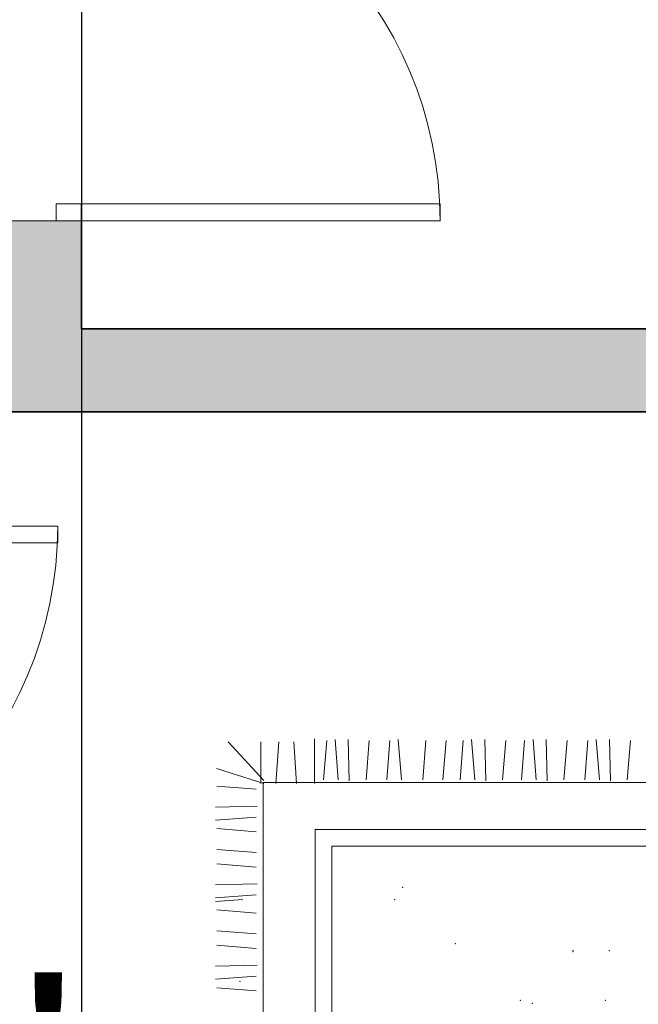
# Model space of a CAD drawing. Units: inches. Extents: x 1763 to 2368, y 1500 to 2097.
# Tile 15 of 24: x 2079 to 2117, y 1797 to 1856. Entities that reach past the tile are written whole.
import ezdxf

# ---------------------------------------------------------------- set-up
doc = ezdxf.new("R2010")
doc.units = ezdxf.units.IN
for name, color, linetype, lineweight in [('A-ANNO-DIMS', 2, 'Continuous', 18), ('A-DOOR', 4, 'Continuous', 18), ('A-FURN', 8, 'Continuous', 18), ('A-WALL', 7, 'Continuous', 35), ('A-WALL-PATT', 7, 'Continuous', 13)]:
    doc.layers.add(name, color=color, linetype=linetype, lineweight=lineweight)
doc.styles.get("Standard").update_dxf_attribs({"font": 'arial.ttf'})
doc.dimstyles.new('ISO-25', dxfattribs={"dimtxt": 12.5, "dimasz": 2.5, "dimexe": 1.25, "dimexo": 0.625, "dimtad": 1, "dimdec": 0, "dimlunit": 4, "dimtxsty": 'Standard', "dimblk": 'ARCHTICK', "dimcen": 2.5, "dimclrd": 3, "dimclrt": 4, "dimadec": 0, "dimazin": 0, "dimtfac": 1, "dimtdec": 0, "dimtmove": 0, "dimatfit": 3, "dimfxl": 1, "dimarcsym": 0})

# ---------------------------------------------------------------- blocks, each defined once
blk = doc.blocks.new('A$C77DF40FE')
for p, q in [((0.1002397472184384, 1.888474420258717), (0.1002397472184384, 0.0935002162950696)), ((0.1852251112431986, 1.811603981208463), (0.1852251112431986, 0.1869505834038136)), ((0.2152251112420345, 1.781603981209627), (0.2152251112420345, 0.2169505834026495)), ((0.0247191405724152, 0.7548065529699671), (0.0955424953790498, 0.7491367263210122)), ((0.0226663125285995, 0.7171728351022466), (0.097390093105787, 0.7188162710299367)), ((0.0226663125285995, 0.6933436513354537), (0.0957477256961283, 0.6990955860601389)), ((0.0247191405724152, 0.6782658048541635), (0.0955424953790498, 0.6725959782124847)), ((0.0247191405724152, 0.6408332608843921), (0.0955424953790498, 0.6351634342354373)), ((0.0226663125285995, 0.6031995430166717), (0.097390093105787, 0.6048429789443617)), ((0.0226663125285995, 0.5793703592498787), (0.0957477256961283, 0.585122293974564)), ((0.0247191405724152, 0.5642925127685885), (0.0955424953790498, 0.5586226861269097)), ((0.0247191405724152, 0.530116254944005), (0.0955424953790498, 0.5244464282950503)), ((0.0226663125285995, 0.4924825370762847), (0.097390093105787, 0.4941259730039747)), ((0.0226663125285995, 0.4686533533094917), (0.0957477256961283, 0.474405288034177)), ((0.0247191405724152, 0.4535755068282015), (0.0955424953790498, 0.4479056801865227)), ((0.0247191405724152, 0.4226553530897946), (0.0955424953790498, 0.4169855264408398)), ((0.0247191405724152, 0.3863853563088924), (0.0955424953790498, 0.3807155296672135)), ((0.0226663125285995, 0.336688923627662), (0.0957477256961283, 0.3424408583450713)), ((0.0247191405724152, 0.3216110771463718), (0.0955424953790498, 0.3159412504974171)), ((0.0247191405724152, 0.2841785331693245), (0.0955424953790498, 0.2785087065203697)), ((0.0226663125285995, 0.2465448153016041), (0.097390093105787, 0.2481882512365701)), ((0.0226663125285995, 0.2227156315420871), (0.0957477256961283, 0.2284675662594964)), ((0.2152251112420345, 0.2169505834026495), (0.3112043679720955, 0.2169505834026495)), ((0.3112043679720955, 0.2169505834026495), (1.613872679183259, 0.2169505834026495)), ((0.0247191405724152, 0.2076377850607969), (0.0955424953790498, 0.2019679584118421)), ((0.1018629931495525, 0.1856925320898881), (0.0215859625604935, 0.1856925320898881)), ((0.1852251112431986, 0.1869505834038136), (0.3112043679720955, 0.1869505834038136)), ((0.3112043679720955, 0.1869505834038136), (1.643872679182095, 0.1869505834038136)), ((0.1018629931495525, 0.153544231550768), (0.0269378679586225, 0.1481852358119795)), ((0.1018629931495525, 0.1160369352728594), (0.0269378679586225, 0.1213930940648424)), ((0.0965110877514235, 0.0946037892645109), (0.0269378679586225, 0.0303071881862707)), ((0.1018629931495525, 0.0892447935257224), (0.0269378679586225, 0.0892447935257224)), ((0.1018629931495525, 0.0946037892645109), (0.0751034661589074, 0.0088740421779221)), ((0.1002397472184384, 0.0935002162950696), (0.3112043679720955, 0.0935002162950696)), ((0.3112043679720955, 0.0935002162950696), (1.015486722324567, 0.0935002162950696)), ((0.1069568759485264, 0.0096009220796986), (0.1126267025974812, 0.0804242768863333)), ((0.1445905938162468, 0.007548094035883), (0.1429471578885568, 0.0822718746130704)), ((0.1684197775830398, 0.007548094035883), (0.1626678428583546, 0.0806295072034118)), ((0.18349762406433, 0.0096009220796986), (0.1891674507060088, 0.0804242768863333)), ((0.2209301680341014, 0.0096009220796986), (0.2265999946830561, 0.0804242768863333)), ((0.2469813674761099, 0.0096009220796986), (0.2526511941250646, 0.0804242768863333)), ((0.2846150853438303, 0.007548094035883), (0.2829716494161403, 0.0822718746130704)), ((0.3084442691106233, 0.007548094035883), (0.302692334385938, 0.0806295072034118)), ((0.3301377238531131, 0.0096009220796986), (0.3358075505020679, 0.0804242768863333)), ((0.3675702678301604, 0.0096009220796986), (0.3732400944791152, 0.0804242768863333)), ((0.3936214672721689, 0.0096009220796986), (0.3992912939211237, 0.0804242768863333)), ((0.4312551851398894, 0.007548094035883), (0.4296117492049234, 0.0822718746130704)), ((0.4550843688994064, 0.007548094035883), (0.4493324341819971, 0.0806295072034118)), ((0.4701622153806966, 0.0096009220796986), (0.4758320420296514, 0.0804242768863333)), ((0.3150598773718229, 0.007548094035883), (0.3112043679720955, 0.0565344072383596))]:
    blk.add_line(p, q)
for p in [(0.4034435357025359, 0.7168515314842808), (0.4931307316510356, 0.7095942980013206), (0.4034435357025359, 0.6511853100746521), (0.4055166808320792, 0.6512242505123141), (0.4983588332761429, 0.5782229147444014), (0.4931307316510356, 0.5563730709764059), (0.3909143693745136, 0.439633238442184), (0.2894910708273528, 0.3447820589062758), (0.3113944469878334, 0.3301895798358601), (0.4588475937125623, 0.0512694676363026)]:
    blk.add_point(p)
blk = doc.blocks.new('*U3')
for p, q in [((0, 0), (-1e-16, -5.999999999999999)), ((40, -6e-16), (40, -6))]:
    blk.add_line(p, q)
blk.add_lwpolyline([(0, 0), (5.6e-15, 40), (1.750000000000007, 40), (1.749999999999998, -7e-16)], close=True)
blk.add_arc((0, 0), 40, 0, 90)
blk = doc.blocks.new('_ArchTick')
at = {"color": 0, "linetype": 'ByBlock', "const_width": 0.15}
blk.add_lwpolyline([(-0.5, -0.5), (0.5, 0.5)], dxfattribs=at)
blk = doc.blocks.new('*D27')
at = {"layer": 'A-ANNO-DIMS', "color": 0, "lineweight": -2, "transparency": 16777216}
for p, q in [((1853.713196592648, 1795.957703707508), (1853.713196592648, 1781.682703707508)), ((1944.713196592648, 1795.957703707508), (1944.713196592648, 1781.682703707508))]:
    blk.add_line(p, q, dxfattribs=at)
at = {"layer": 'A-ANNO-DIMS', "color": 3, "lineweight": -2, "transparency": 16777216}
for p, q in [((1853.713196592648, 1782.932703707508), (1944.713196592648, 1782.932703707508)), ((1944.713196592648, 1782.932703707508), (2085.85235075363, 1782.932703707508))]:
    blk.add_line(p, q, dxfattribs=at)
at = {"layer": 'Defpoints', "color": 0, "transparency": 16777216}
for p in [(1853.713196592648, 1796.582703707508), (1944.713196592648, 1796.582703707508), (1944.713196592648, 1782.932703707508)]:
    blk.add_point(p, dxfattribs=at)
at = {"layer": 'A-ANNO-DIMS', "color": 3, "lineweight": -2, "transparency": 16777216, "xscale": 2.5, "yscale": 2.5, "zscale": 2.5, "rotation": 180}
blk.add_blockref('_ArchTick', (1853.713196592648, 1782.932703707508), dxfattribs=at)
at = {"layer": 'A-ANNO-DIMS', "color": 3, "lineweight": -2, "transparency": 16777216, "xscale": 2.5, "yscale": 2.5, "zscale": 2.5}
blk.add_blockref('_ArchTick', (1944.713196592648, 1782.932703707508), dxfattribs=at)
at = {"layer": 'A-ANNO-DIMS', "color": 4, "transparency": 16777216, "insert": (2016.532773673139, 1790.020868782542), "char_height": 12.5, "attachment_point": 5}
blk.add_mtext('DINING SET 7\'-7"', dxfattribs=at)
blk = doc.blocks.new('*D62')
at = {"layer": 'A-ANNO-DIMS', "color": 0, "lineweight": -2, "transparency": 16777216}
for p, q in [((2083.09181, 1980.647691), (2083.09181, 1509.906119)), ((2120.612101, 1980.647691), (2120.612101, 1509.906119))]:
    blk.add_line(p, q, dxfattribs=at)
at = {"layer": 'A-ANNO-DIMS', "color": 3, "lineweight": -2, "transparency": 16777216}
for p, q in [((2083.09181, 1511.156119), (2120.612101, 1511.156119)), ((2120.612101, 1511.156119), (2186.708622145976, 1511.156119))]:
    blk.add_line(p, q, dxfattribs=at)
at = {"layer": 'Defpoints', "color": 0, "transparency": 16777216}
for p in [(2083.09181, 1981.272691), (2120.612101, 1981.272691), (2120.612101, 1511.156119)]:
    blk.add_point(p, dxfattribs=at)
at = {"layer": 'A-ANNO-DIMS', "color": 3, "lineweight": -2, "transparency": 16777216, "xscale": 2.5, "yscale": 2.5, "zscale": 2.5, "rotation": 180}
blk.add_blockref('_ArchTick', (2083.09181, 1511.156119), dxfattribs=at)
at = {"layer": 'A-ANNO-DIMS', "color": 3, "lineweight": -2, "transparency": 16777216, "xscale": 2.5, "yscale": 2.5, "zscale": 2.5}
blk.add_blockref('_ArchTick', (2120.612101, 1511.156119), dxfattribs=at)
at = {"layer": 'A-ANNO-DIMS', "color": 4, "transparency": 16777216, "insert": (2154.910361572988, 1518.248547376535), "char_height": 12.5, "attachment_point": 5}
blk.add_mtext('3\'-1 1/2"', dxfattribs=at)
blk = doc.blocks.new('*D71')
at = {"layer": 'A-ANNO-DIMS', "color": 0, "lineweight": -2, "transparency": 16777216}
for p, q in [((2049.685769, 1879.647691), (2049.685769, 1509.906119)), ((2072.784807, 1879.647691), (2072.784807, 1509.906119))]:
    blk.add_line(p, q, dxfattribs=at)
at = {"layer": 'A-ANNO-DIMS', "color": 3, "lineweight": -2, "transparency": 16777216}
for p, q in [((2049.685769, 1511.156119), (2072.784807, 1511.156119)), ((2072.784807, 1511.156119), (2118.298108500682, 1511.156119))]:
    blk.add_line(p, q, dxfattribs=at)
at = {"layer": 'Defpoints', "color": 0, "transparency": 16777216}
for p in [(2049.685769, 1880.272691), (2072.784807, 1880.272691), (2072.784807, 1511.156119)]:
    blk.add_point(p, dxfattribs=at)
at = {"layer": 'A-ANNO-DIMS', "color": 3, "lineweight": -2, "transparency": 16777216, "xscale": 2.5, "yscale": 2.5, "zscale": 2.5, "rotation": 180}
blk.add_blockref('_ArchTick', (2049.685769, 1511.156119), dxfattribs=at)
at = {"layer": 'A-ANNO-DIMS', "color": 3, "lineweight": -2, "transparency": 16777216, "xscale": 2.5, "yscale": 2.5, "zscale": 2.5}
blk.add_blockref('_ArchTick', (2072.784807, 1511.156119), dxfattribs=at)
at = {"layer": 'A-ANNO-DIMS', "color": 4, "transparency": 16777216, "insert": (2096.791457750341, 1518.056698809004), "char_height": 12.5, "attachment_point": 5}
blk.add_mtext('1\'-11"', dxfattribs=at)

msp = doc.modelspace()

# ---------------------------------------------------------------- hatches: boundary and pattern name
at = {"layer": 'A-WALL-PATT'}
h = msp.add_hatch(color=256, dxfattribs=at)
h.dxf.hatch_style = 1
h.paths.add_polyline_path([(1838.091809557101, 2034.272690883634), (1838.091809557101, 2043.272690883634), (1829.091809557101, 2043.272690883634), (1829.091809557101, 1953.387436665241), (1838.091809557101, 1953.387436665241)])
h.paths.add_polyline_path([(1838.091809557101, 1913.100906919557), (1829.091809557101, 1913.100906919557), (1829.091809557101, 1862.201751012257), (1838.091809557101, 1862.201751012257)])
h.paths.add_polyline_path([(1838.091809557101, 1825.58961200371), (1829.091809557101, 1825.58961200371), (1829.091809557101, 1738.643388462881), (1838.091809557101, 1738.643388462881)])
h.paths.add_polyline_path([(1895.591809557102, 1885.272690883634), (1838.091809557101, 1885.272690883634), (1838.091809557101, 1880.272690883634), (1895.591809557102, 1880.272690883634)])
h.paths.add_polyline_path([(1857.388795027446, 1784.272690883634), (1838.091809557101, 1784.272690883634), (1838.091809557101, 1779.272690883634), (1857.388795027446, 1779.272690883634)])
h.paths.add_polyline_path([(1958.091809557101, 1981.272690883634), (1971.455231199137, 1981.272690883634), (1971.455231199137, 1986.272690883634), (1968.567697615106, 1986.272690883634), (1958.091809557101, 1986.272690883634), (1953.091809557101, 1986.272690883634), (1927.390355781482, 1986.272690883634), (1927.390355781482, 1981.272690883634), (1953.091809557102, 1981.272690883634), (1953.091809557102, 1885.272690883634), (1932.013525308711, 1885.272690883634), (1932.013525308711, 1880.272690883634), (1959.134211901633, 1880.272690883634), (1959.134211901633, 1883.737546537067), (1959.134211901633, 1885.272690883634), (1958.091809557101, 1885.272690883634)])
h.paths.add_polyline_path([(2018.091809557102, 1981.272690883634), (2031.018823922628, 1981.272690883634), (2031.018823922628, 1986.272690883634), (2018.091809557102, 1986.272690883634), (2013.091809557101, 1986.272690883634), (2001.2328901763, 1986.272690883634), (2001.2328901763, 1981.272690883634), (2013.091809557101, 1981.272690883634), (2013.091809557101, 1885.272690883634), (1982.182180879804, 1885.272690883634, -0.0166285960272348), (1982.233249591189, 1883.737546537067), (1982.233249591189, 1880.272690883634), (2049.685769014253, 1880.272690883634), (2049.685769014253, 1883.737546537067, -0.0166285960272329), (2049.736837725638, 1885.272690883634), (2018.091809557102, 1885.272690883634)])
h.paths.add_polyline_path([(2083.091809557101, 1981.272690883633), (2120.612101449853, 1981.272690883633), (2120.612101449853, 1986.272690883634), (2083.091809557101, 1986.272690883634), (2078.091809557101, 1986.272690883634), (2063.142597715185, 1986.272690883634), (2063.142597715185, 1981.272690883634), (2078.091809557101, 1981.272690883634), (2078.091809557101, 1885.272690883634), (2072.784806703809, 1885.272690883634), (2072.784806703809, 1883.737546537067), (2072.784806703809, 1880.272690883634), (2078.091809557101, 1880.272690883634), (2078.091809557101, 1866.867159403521), (2081.556665210535, 1866.867159403521, -0.0166285960272329), (2083.091809557101, 1866.816090692136)])
h.paths.add_polyline_path([(1871.675401748104, 1635.272690883634), (1838.091809557101, 1635.272690883634), (1838.091809557101, 1626.272690883634), (1871.675401748104, 1626.272690883634)], flags=17)
h.paths.add_polyline_path([(2100.577130801176, 1688.272690883634), (2060.091809557102, 1688.272690883634), (2060.091809557102, 1679.272690883634), (2100.577130801176, 1679.272690883634)], flags=17)
h.paths.add_polyline_path([(2180.091809557101, 1688.272690883634), (2148.743529320587, 1688.272690883634), (2148.743529320587, 1679.272690883634), (2180.091809557101, 1679.272690883634)], flags=17)
h.paths.add_polyline_path([(2189.091809557101, 1746.219079973147), (2180.091809557101, 1746.219079973147), (2180.091809557101, 1743.41673524497), (2180.123283967846, 1743.41673524497), (2180.123283967846, 1726.723261858881), (2180.091809557101, 1572.272690883634), (2034.906803433656, 1572.272690883634), (2034.906803433656, 1565.600894774026), (2034.906803433656, 1563.272690883634), (2189.091809557101, 1563.272690883634)])
h.paths.add_polyline_path([(2060.091809557102, 1802.347155552507, -0.0166285960272347), (2058.556665210535, 1802.296086841122), (2055.091809557101, 1802.296086841122), (2055.091809557101, 1635.272690883634), (2042.484481853934, 1635.272690883634), (2042.484481853934, 1629.737546537067), (2042.484481853934, 1626.272690883634), (2055.091809557101, 1626.272690883634), (2055.091809557101, 1599.272690883634), (2040.268709306729, 1599.272690883634), (2040.268709306729, 1590.272690883634), (2060.091809557102, 1590.272690883634)])
h.paths.add_polyline_path([(2019.385444164378, 1629.737546537071, -0.0605692182813801), (2020.058431839583, 1635.272690883634), (1995.091809557101, 1635.272690883634), (1990.091809557101, 1635.272690883634), (1927.074869319207, 1635.272690883634), (1927.074869319207, 1626.272690883634), (1990.091809557101, 1626.272690883634), (1990.091809557102, 1590.272690883634), (1995.091809557101, 1590.272690883634), (2005.195459372391, 1590.272690883634), (2005.195459372391, 1599.272690883634), (1995.091809557101, 1599.272690883634), (1995.091809557101, 1626.272690883634), (2019.385444164378, 1626.272690883634)])
edge = h.paths.add_edge_path()
edge.add_line((2180.091809557101, 1837.272690883634), (2167.198417694339, 1837.272690883634))
edge.add_spline(control_points=[(2167.198417694823, 1837.272690883674), (2167.1907827488, 1837.271431447654), (2167.183204353112, 1837.271421440364), (2167.175683403496, 1837.272690883654)], knot_values=[168.9554928085609, 168.9554928085609, 168.9554928085609, 168.9554928085609, 169.0658706879006, 169.0658706887506, 169.0658706887506, 169.0658706887506], degree=3, periodic=0)
edge.add_spline(control_points=[(2167.175683403438, 1837.272690883663), (2166.556253545484, 1837.377242984508), (2166.326495733136, 1846.160649987724), (2165.707502931977, 1846.244137993658)], knot_values=[159.864705322856, 159.8647053237059, 159.8647053237059, 159.8647053237059, 168.9554928094108, 168.9554928094108, 168.9554928094108, 168.9554928094108], degree=3, periodic=0)
edge.add_line((2167.122451608289, 1837.272690883634), (2163.159522476786, 1837.272690883634))
edge.add_spline(control_points=[(2163.159522482475, 1837.272690883686), (2163.15796606182, 1837.2726620788), (2163.156410184994, 1837.272662044343), (2163.15485485529, 1837.272690883634)], knot_values=[150.5371721295467, 150.5371721295467, 150.5371721295467, 150.5371721295467, 150.5537966479016, 150.5537966479139, 150.5537966479139, 150.5537966479139], degree=3, periodic=0)
edge.add_spline(control_points=[(2163.154854855289, 1837.272690883634), (2162.290043487653, 1837.288726420245), (2161.594386529693, 1846.231668717186), (2160.877825059406, 1846.244137993679)], knot_values=[141.2934262950179, 141.2934262950303, 141.2934262950303, 141.2934262950303, 150.5371721295591, 150.5371721295591, 150.5371721295591, 150.5371721295591], degree=3, periodic=0)
edge.add_line((2163.075401221166, 1837.272690883634), (2158.699619590683, 1837.272690883634))
edge.add_spline(control_points=[(2158.6996195907, 1837.272690883634), (2158.698397652875, 1837.272665391618), (2158.697175755076, 1837.272665420255), (2158.695953896478, 1837.272690883674)], knot_values=[132.0335441852708, 132.0335441852708, 132.0335441852708, 132.0335441852771, 132.0491510388534, 132.0491510388534, 132.0491510388534, 132.0491510388534], degree=3, periodic=0)
edge.add_spline(control_points=[(2158.695953896478, 1837.272690883674), (2157.971966468073, 1837.287778714179), (2157.261742058153, 1846.232799164874), (2156.393385429706, 1846.244137993689)], knot_values=[122.7860209386129, 122.7860209386129, 122.7860209386129, 122.7860209386129, 132.0335441852594, 132.0335441852594, 132.0335441852594, 132.0335441852708], degree=3, periodic=0)
edge.add_line((2158.629450057908, 1837.272690883634), (2153.839354197273, 1837.272690883634))
edge.add_spline(control_points=[(2153.839354197267, 1837.272690883633), (2153.831393241206, 1837.271421595935), (2153.823483829624, 1837.271411470755), (2153.815626850732, 1837.272690883634)], knot_values=[113.4515845582001, 113.4515845582001, 113.4515845582001, 113.4515845582001, 113.5621029574639, 113.5621029574639, 113.5621029574639, 113.5621029574668], degree=3, periodic=0)
edge.add_spline(control_points=[(2153.815626850732, 1837.272690883634), (2153.16997926524, 1837.3778266931), (2152.878395890465, 1846.19087494863), (2152.403814355283, 1846.244137993689)], knot_values=[0, 0, 0, 0, 9.081854313454823, 9.081854313454823, 9.081854313454823, 9.081854313454823], degree=3, periodic=0)
edge.add_line((2153.760174359353, 1837.272690883634), (2150.390681228399, 1837.272690883634))
edge.add_spline(control_points=[(2150.390681228397, 1837.272690883634), (2150.380731407352, 1837.271531119858), (2150.370755552885, 1837.271539860845), (2150.360754310833, 1837.272690883655)], knot_values=[95.0693824194044, 95.0693824194044, 95.0693824194044, 95.06938241940794, 95.17519011295934, 95.17519011295934, 95.17519011295934, 95.17519011295934], degree=3, periodic=0)
edge.add_spline(control_points=[(2150.360754310833, 1837.272690883655), (2149.486911233016, 1837.373259724043), (2148.41925626668, 1846.194145922126), (2147.588575190972, 1846.244137993689)], knot_values=[85.8245986104526, 85.8245986104526, 85.8245986104526, 85.8245986104526, 95.06938241940442, 95.06938241940442, 95.06938241940442, 95.06938241940442], degree=3, periodic=0)
edge.add_line((2150.286144937881, 1837.272690883634), (2145.429521599744, 1837.272690883634))
edge.add_spline(control_points=[(2145.429521599744, 1837.272690883634), (2145.426173195383, 1837.272505952667), (2145.422821785984, 1837.272506511139), (2145.419467387339, 1837.272690883634)], knot_values=[76.50555885182466, 76.50555885182466, 76.50555885182466, 76.50555885182986, 76.54781121413636, 76.54781121413636, 76.54781121413636, 76.54781121413636], degree=3, periodic=0)
edge.add_spline(control_points=[(2145.419467387339, 1837.272690883634), (2144.683834601378, 1837.313124495274), (2143.804436376202, 1846.193948544996), (2142.947843667561, 1846.244137993688)], knot_values=[67.23944999382844, 67.23944999382844, 67.23944999382844, 67.23944999382844, 76.50555885179328, 76.50555885179328, 76.50555885179328, 76.50555885182465], degree=3, periodic=0)
edge.add_line((2145.353375417295, 1837.272690883634), (2134.569944747806, 1837.272690883634))
edge.add_spline(control_points=[(2134.56994474779, 1837.272690883634), (2134.566672918288, 1837.272498574207), (2134.563405957571, 1837.27249916596), (2134.560143779651, 1837.272690883636)], knot_values=[39.00146280124788, 39.00146280124788, 39.00146280124788, 39.00146280126319, 39.04510672327663, 39.04510672327663, 39.04510672327663, 39.04510672327663], degree=3, periodic=0)
edge.add_spline(control_points=[(2134.560143779651, 1837.272690883636), (2133.872211796742, 1837.313120536706), (2133.396974976361, 1845.853088067863), (2132.328029807564, 1846.244137993689)], knot_values=[29.79778030706209, 29.79778030706209, 29.79778030706209, 29.79778030706209, 39.00146280124655, 39.00146280124788, 39.00146280124788, 39.00146280124788], degree=3, periodic=0)
edge.add_line((2134.498286803723, 1837.272690883634), (2128.075271300648, 1837.272690883634))
edge.add_spline(control_points=[(2128.075271300648, 1837.272690883634), (2128.026285766884, 1837.259723584904), (2127.978195692325, 1837.26004073722), (2127.930927784897, 1837.272690883634)], knot_values=[19.48206652474599, 19.48206652474599, 19.48206652474599, 19.48206652474654, 19.86939583794397, 19.86939583794397, 19.86939583794397, 19.86939583794397], degree=3, periodic=0)
edge.add_spline(control_points=[(2125.013283184744, 1846.244137993688), (2126.164818330763, 1844.662568162717), (2126.821349600389, 1837.569643451595), (2127.930927784897, 1837.272690883634)], knot_values=[10.38980542113492, 10.3898054211352, 10.3898054211352, 10.3898054211352, 19.48206652474599, 19.48206652474599, 19.48206652474599, 19.48206652474599], degree=3, periodic=0)
edge.add_line((2127.930927784898, 1837.272690883634), (2083.091809557101, 1837.272690883634))
edge.add_line((2083.091809557101, 1837.272690883634), (2083.091809557101, 1843.768121713965))
edge.add_line((2083.091809557101, 1843.768121713965), (2081.556665210535, 1843.768121713965))
edge.add_line((2081.556665210535, 1843.768121713965), (2078.091809557101, 1843.768121713965))
edge.add_line((2078.091809557101, 1843.768121713965), (2078.091809557101, 1837.272690883634))
edge.add_line((2078.091809557101, 1837.272690883634), (2055.091809557101, 1837.272690883634))
edge.add_line((2055.091809557101, 1837.272690883634), (2055.091809557101, 1825.395124530677))
edge.add_line((2055.091809557101, 1825.395124530677), (2058.556665210535, 1825.395124530677))
edge.add_line((2058.556665210535, 1825.395124530677), (2060.091809557102, 1825.395124530677))
edge.add_line((2060.091809557102, 1825.395124530677), (2060.091809557102, 1832.272690883634))
edge.add_line((2060.091809557102, 1832.272690883634), (2122.436734598602, 1832.272690883634))
edge.add_spline(control_points=[(2122.436734598601, 1832.272690883634), (2122.727456143255, 1832.584305259818), (2123.008062474702, 1832.616792422395), (2123.275021713284, 1832.272690883634)], knot_values=[5.972032537224317, 5.972032537224317, 5.972032537224317, 5.972032537224317, 8.057258009602386, 8.057258009602837, 8.057258009602837, 8.057258009602837], degree=3, periodic=0)
edge.add_line((2123.275021713284, 1832.272690883634), (2137.951393308032, 1832.272690883634))
edge.add_spline(control_points=[(2137.951393307966, 1832.272690883629), (2137.961042543445, 1832.274026104781), (2137.970676309981, 1832.27403826157), (2137.980294423909, 1832.272690883634)], knot_values=[53.92686179676418, 53.92686179676418, 53.92686179676418, 53.92686179676418, 54.03007548000314, 54.03007548000314, 54.03007548000314, 54.03007548000601], degree=3, periodic=0)
edge.add_spline(control_points=[(2139.715582741171, 1825.016325920323), (2139.281482802356, 1825.062086475526), (2138.671282749905, 1832.175892027703), (2137.98029442391, 1832.272690883634)], knot_values=[54.03007548000314, 54.03007548000314, 54.03007548000314, 54.03007548000314, 61.44519353062353, 61.44519353062641, 61.44519353062641, 61.44519353062641], degree=3, periodic=0)
edge.add_line((2138.045183132032, 1832.272690883634), (2140.961787078569, 1832.272690883634))
edge.add_spline(control_points=[(2140.96178707854, 1832.272690883628), (2140.970606368947, 1832.274440590632), (2140.979501539198, 1832.27442261757), (2140.988470957723, 1832.272690883634)], knot_values=[68.85418231261454, 68.85418231261454, 68.85418231261454, 68.85418231280003, 68.97123731673409, 68.97123731673409, 68.97123731673409, 68.97123731673409], degree=3, periodic=0)
edge.add_spline(control_points=[(2143.18986511145, 1825.016325920314), (2142.436495288906, 1825.065396856983), (2141.561146249046, 1832.16212393513), (2140.988470957723, 1832.272690883634)], knot_values=[68.9712373167341, 68.97123731708082, 68.97123731708082, 68.97123731708082, 76.44491114487315, 76.44491114487315, 76.44491114487315, 76.44491114487315], degree=3, periodic=0)
edge.add_line((2141.040932085754, 1832.272690883634), (2145.429521599744, 1832.272690883634))
edge.add_spline(control_points=[(2145.429521599742, 1832.272690883634), (2145.43886220747, 1832.273579662711), (2145.448227241903, 1832.27357314134), (2145.457616067813, 1832.272690883634)], knot_values=[84.03904662338796, 84.03904662338796, 84.03904662338796, 84.03904662338971, 84.12404068496751, 84.12404068496751, 84.12404068496751, 84.12404068496751], degree=3, periodic=0)
edge.add_spline(control_points=[(2148.107765738118, 1825.016325920317), (2147.340420200817, 1825.019697773855), (2146.30265295, 1832.193283691691), (2145.457616067813, 1832.272690883634)], knot_values=[84.12404068496751, 84.12404068496751, 84.12404068496751, 84.12404068496751, 91.77389142141917, 91.77389142141917, 91.77389142141917, 91.77389142141917], degree=3, periodic=0)
edge.add_line((2145.537886823607, 1832.272690883634), (2150.392945902062, 1832.272690883634))
edge.add_spline(control_points=[(2150.392945902064, 1832.272690883634), (2150.41883348599, 1832.27702102203), (2150.445058688081, 1832.276951395392), (2150.471602715227, 1832.272690883634)], knot_values=[99.38157707204087, 99.3815770720414, 99.3815770720414, 99.3815770720414, 99.57345662964875, 99.57345662964875, 99.57345662964875, 99.57345662964875], degree=3, periodic=0)
edge.add_spline(control_points=[(2153.974048108825, 1825.016325920308), (2153.092849423049, 1825.280585632922), (2151.529174697084, 1832.102942795321), (2150.471602715227, 1832.272690883634)], knot_values=[99.57345662964875, 99.57345662964875, 99.57345662964875, 99.57345662964875, 107.2183570397887, 107.2183570397887, 107.2183570397887, 107.2183570397887], degree=3, periodic=0)
edge.add_line((2150.568426065927, 1832.272690883634), (2155.598049458685, 1832.272690883634))
edge.add_spline(control_points=[(2155.59804945868, 1832.272690883633), (2155.604650662926, 1832.273493563234), (2155.611310013868, 1832.273487964753), (2155.618026602473, 1832.272690883629)], knot_values=[114.9330576886776, 114.9330576886776, 114.9330576886776, 114.9330576886986, 115.0136243763172, 115.0136243763172, 115.0136243763172, 115.0136243763172], degree=3, periodic=0)
edge.add_spline(control_points=[(2158.284655371249, 1825.016325920309), (2157.395326401988, 1825.074357796858), (2156.251834921329, 1832.197474627747), (2155.618026602473, 1832.272690883629)], knot_values=[115.0136243763171, 115.0136243763171, 115.0136243763171, 115.0136243763171, 122.6162690869638, 122.6162690869638, 122.6162690869638, 122.6162690869638], degree=3, periodic=0)
edge.add_line((2155.677997005666, 1832.272690883634), (2165.194843181567, 1832.272690883634))
edge.add_spline(control_points=[(2165.194843180774, 1832.272690883621), (2165.197973141718, 1832.272787704364), (2165.201103815629, 1832.272787940576), (2165.204235204227, 1832.27269088363)], knot_values=[145.4884769441583, 145.4884769441583, 145.4884769441583, 145.4884769441583, 145.5163785292906, 145.5163785298517, 145.5163785298517, 145.5163785298517], degree=3, periodic=0)
edge.add_spline(control_points=[(2167.445935353137, 1825.016325920312), (2166.960552374007, 1825.022023955429), (2166.055957046383, 1832.246291885329), (2165.204235204289, 1832.272690883628)], knot_values=[145.5163785292906, 145.5163785292906, 145.5163785292906, 145.5163785292906, 153.1054685509886, 153.1054685509886, 153.1054685509886, 153.1054685515498], degree=3, periodic=0)
edge.add_line((2165.289510410991, 1832.272690883634), (2168.928217296476, 1832.272690883634))
edge.add_spline(control_points=[(2168.928217296468, 1832.272690883631), (2168.9815111362, 1832.293215999779), (2169.037604970232, 1832.292507987016), (2169.096218703475, 1832.272690883634)], knot_values=[160.5174393135676, 160.5174393135676, 160.5174393135676, 160.5174393135912, 160.9397230621378, 160.9397230621378, 160.9397230621378, 160.9397230621378], degree=3, periodic=0)
edge.add_spline(control_points=[(2171.08610288907, 1828.644508401971), (2170.354822507508, 1830.369456517115), (2169.623542125945, 1832.094404632258), (2169.096218703475, 1832.272690883634)], knot_values=[160.9397230621378, 160.9397230621378, 160.9397230621378, 160.9397230621378, 164.7388346221332, 164.7388346221332, 164.7388346221332, 164.7388346221332], degree=3, periodic=0)
edge.add_line((2169.096218703475, 1832.272690883634), (2180.091809557101, 1832.272690883634))
edge.add_line((2180.091809557101, 1832.272690883634), (2180.091809557101, 1837.272690883634))
h.paths.add_polyline_path([(2189.091809557101, 1885.522968548043), (2180.091809557101, 1885.522968548043), (2180.091809557101, 1813.316873906924), (2180.123283967846, 1813.316873906924), (2180.123283967846, 1796.623400520835), (2180.123092181994, 1795.256344207559), (2189.091809557101, 1795.256344207559)])
h.paths.add_polyline_path([(2180.091809557101, 1986.272690883634), (2166.279557011185, 1986.272690883634), (2166.279557011185, 1981.272690883634), (2180.091809557101, 1981.272690883634)])
h.paths.add_polyline_path([(2189.091809557101, 2043.272690883634), (2180.091809557101, 2043.272690883634), (2180.091809557101, 2034.272690883634), (2180.091809557101, 1934.108443350786), (2189.091809557101, 1934.108443350786)])
h.paths.add_polyline_path([(1838.091809557101, 1681.591873076235), (1829.091809557101, 1681.591873076235), (1829.091809557101, 1563.272690883634), (2003.864084895099, 1563.272690883634), (2003.864084895099, 1565.600894774026), (2003.864084895099, 1572.272690883634), (1838.091809557101, 1572.272690883634)])

# ---------------------------------------------------------------- linework, layer by layer
at = {"layer": 'A-WALL'}
for p, q in [((2083.091809557101, 1837.272690883634), (2083.091809557101, 1844.778704612883)), ((2083.091809557101, 1837.272690883634), (2180.091809557101, 1837.272690883634)), ((2060.091809557102, 1832.272690883634), (2180.091809557101, 1832.272690883634))]:
    msp.add_line(p, q, dxfattribs=at)

# ---------------------------------------------------------------- block references
at = {"layer": 'A-DOOR', "yscale": 0.5774759422388936, "zscale": 0.5774759422388936, "rotation": 270}
for p, xscale in [((2081.556665210535, 1843.768121713965), -0.5774759422388936), ((2058.556665210535, 1825.395124530677), 0.5774759422388936)]:
    msp.add_blockref('*U3', p, dxfattribs=dict(at, xscale=xscale))
at = {"layer": 'A-FURN', "xscale": 33.38694677217886, "yscale": 33.38694677217886, "zscale": 33.38694677217886, "rotation": 270}
msp.add_blockref('A$C77DF40FE', (2090.901844803704, 1813.316873335329), dxfattribs=at)

# ---------------------------------------------------------------- dimensions: what is measured, and where the dimension line sits
at = {"layer": 'A-ANNO-DIMS'}
for base, p1, p2, picture, middle in [((2120.612101, 1511.156119), (2083.09181, 1981.272691), (2120.612101, 1981.272691), '*D62', (2154.910361572988, 1518.248547376535)), ((2072.784807, 1511.156119), (2049.685769, 1880.272691), (2072.784807, 1880.272691), '*D71', (2096.791457750341, 1518.056698809004))]:
    dim = msp.add_linear_dim(base=base, p1=p1, p2=p2, dimstyle='ISO-25', override={"dimdec": 1, "dimlfac": 1, "dimrnd": 0, "dimzin": 1, "dimdsep": 46, "dimlunit": 4, "dimfrac": 2}, dxfattribs=at)
    dim.commit()
    dim.dimension.update_dxf_attribs({"geometry": picture, "text_midpoint": middle})
dim = msp.add_linear_dim(base=(1944.713196592648, 1782.932703707508), p1=(1853.713196592648, 1796.582703707508), p2=(1944.713196592648, 1796.582703707508), text='DINING SET <>', dimstyle='ISO-25', override={"dimdec": 1, "dimlfac": 1, "dimrnd": 0, "dimzin": 1, "dimdsep": 46, "dimlunit": 4, "dimfrac": 2}, dxfattribs=at)
dim.commit()
dim.dimension.update_dxf_attribs({"geometry": '*D27', "text_midpoint": (2016.532773673139, 1790.020868782542)})

doc.saveas('drawing.dxf')
